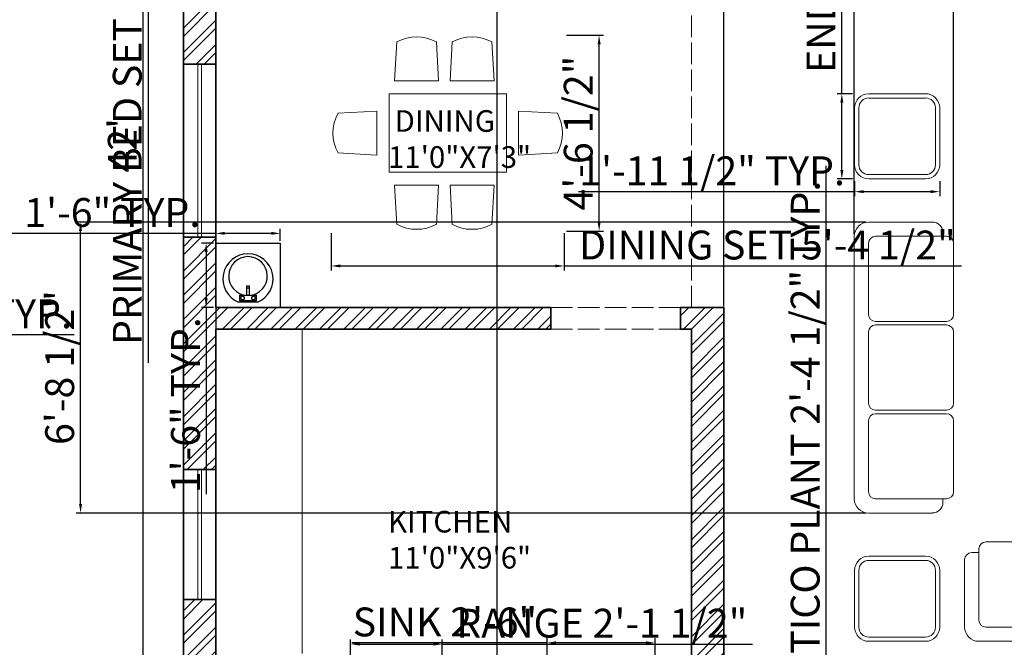
# Model space of a CAD drawing. Units: inches. Extents: x 3595 to 4516, y 2363 to 2965.
# Tile 7 of 12: x 4036 to 4309, y 2512 to 2686. Entities that reach past the tile are written whole.
import ezdxf

# ---------------------------------------------------------------- set-up
doc = ezdxf.new("R2010")
doc.units = ezdxf.units.IN
doc.linetypes.add('ACAD_ISO02W100', pattern=[15, 12, -3])
for name, color, linetype, lineweight in [('A-ANNO-DIMS', 2, 'Continuous', 18), ('A-AREA-IDEN', 7, 'Continuous', 18), ('A-FLOR-CASE', 9, 'Continuous', 18), ('A-FLOR-FIXT', 8, 'Continuous', 18), ('A-FURN', 43, 'Continuous', 18), ('A-GLAZ', 4, 'Continuous', 18), ('A-WALL', 7, 'Continuous', 35), ('A-WALL-OVHD', 7, 'ACAD_ISO02W100', 18)]:
    doc.layers.add(name, color=color, linetype=linetype, lineweight=lineweight)
doc.layers.add('A-WALL-PATT', color=251, linetype='Continuous', lineweight=13, true_color=0x636466)
doc.layers.add('SANTEH', color=7, linetype='Continuous')
doc.styles.get("Standard").update_dxf_attribs({"font": 'arial.ttf'})
doc.dimstyles.new('ISO-25', dxfattribs={"dimtxt": 8, "dimasz": 2.5, "dimexe": 1.25, "dimexo": 0.625, "dimtad": 1, "dimdec": 1, "dimlunit": 3, "dimtxsty": 'Standard', "dimcen": 2.5, "dimadec": 0, "dimazin": 0, "dimtfac": 1, "dimtdec": 1, "dimtmove": 0, "dimatfit": 3, "dimfxl": 1, "dimarcsym": 0})

# ---------------------------------------------------------------- blocks, each defined once
blk = doc.blocks.new('*D6')
at = {"layer": 'A-ANNO-DIMS', "color": 0, "lineweight": -2, "transparency": 16777216}
for p, q in [((4080.62, 2903.04), (4068.71, 2903.04)), ((4069.96, 2900.54), (4069.96, 2401.54)), ((4080.62, 2399.04), (4068.71, 2399.04))]:
    blk.add_line(p, q, dxfattribs=at)
at = {"layer": 'A-ANNO-DIMS', "color": 0, "transparency": 16777216}
for points in [[(4069.55, 2900.54), (4070.38, 2900.54), (4069.96, 2903.04)], [(4069.55, 2401.54), (4070.38, 2401.54), (4069.96, 2399.04)]]:
    blk.add_solid(points, dxfattribs=at)
at = {"layer": 'Defpoints', "color": 0, "transparency": 16777216}
for p in [(4081.24, 2903.04), (4069.96, 2399.04), (4081.24, 2399.04)]:
    blk.add_point(p, dxfattribs=at)
at = {"layer": 'A-ANNO-DIMS', "color": 0, "transparency": 16777216, "insert": (4065.32, 2651.04), "char_height": 8, "attachment_point": 5, "rotation": 90}
blk.add_mtext("42'", dxfattribs=at)
blk = doc.blocks.new('table-11')
at = {"color": 0, "linetype": 'ByBlock'}
for p, q in [((-1.122, 0.533), (-1.144, 0.134)), ((-0.716, 0.533), (-0.694, 0.134)), ((-0.554, 0.533), (-0.576, 0.134)), ((-0.148, 0.533), (-0.126, 0.134)), ((-1.144, 0.134), (-0.694, 0.134)), ((-0.576, 0.134), (-0.126, 0.134)), ((0, 0), (-1.2, 0)), ((-1.2, -0.8), (-1.2, 0)), ((0, -0.8), (0, 0)), ((-1.723, -0.197), (-1.324, -0.175)), ((-1.324, -0.625), (-1.324, -0.175)), ((0.523, -0.197), (0.124, -0.175)), ((0.124, -0.625), (0.124, -0.175)), ((-1.723, -0.603), (-1.324, -0.625)), ((0.523, -0.603), (0.124, -0.625)), ((0, -0.8), (-1.2, -0.8)), ((-1.144, -0.934), (-0.694, -0.934)), ((-1.122, -1.333), (-1.144, -0.934)), ((-0.716, -1.333), (-0.694, -0.934)), ((-0.576, -0.934), (-0.126, -0.934)), ((-0.554, -1.333), (-0.576, -0.934)), ((-0.148, -1.333), (-0.126, -0.934))]:
    blk.add_line(p, q, dxfattribs=at)
for centre, start, end in [((-0.919, 0.159), 61.4891, 118.5109), ((-0.351, 0.159), 61.4891, 118.5109), ((-1.349, -0.4), 151.4891, 208.5109), ((0.149, -0.4), 331.4891, 28.5109), ((-0.919, -0.959), 241.4891, 298.5109), ((-0.351, -0.959), 241.4891, 298.5109)]:
    blk.add_arc(centre, 0.425, start, end, dxfattribs=at)
blk = doc.blocks.new('r11')
at = {"layer": 'SANTEH', "ltscale": 5}
for p, q in [((0, 0), (600, 0)), ((0, -600), (0, 0)), ((600, 0), (600, -600)), ((210.5, -50), (389.5, -50)), ((210.5, -50), (210.5, -50)), ((223.8, -63.2), (376.2, -63.2)), ((223.8, -113.2), (223.8, -63.2)), ((232.7, -78.7), (249.2, -69.1)), ((232.7, -97.7), (232.7, -78.7)), ((249.2, -69.1), (265.7, -78.7)), ((265.7, -78.7), (265.7, -97.7)), ((334.3, -78.7), (350.8, -69.1)), ((334.3, -97.7), (334.3, -78.7)), ((350.8, -69.1), (367.3, -78.7)), ((367.3, -78.7), (367.3, -97.7)), ((376.2, -63.2), (376.2, -113.2)), ((376.2, -113.2), (223.8, -113.2)), ((249.2, -107.2), (232.7, -97.7)), ((265.7, -97.7), (249.2, -107.2)), ((288, -201.6), (288, -113.2)), ((312, -113.2), (312, -201.6)), ((350.8, -107.2), (334.3, -97.7)), ((367.3, -97.7), (350.8, -107.2)), ((312, -184.3), (288, -184.3)), ((312, -201.6), (288, -201.6)), ((600, -600), (0, -600))]:
    blk.add_line(p, q, dxfattribs=at)
for centre, radius, start, end in [((300, -266.2), 234, 112.50001, 67.49999), ((300, -293), 180.2, 93.8183, 86.1817)]:
    blk.add_arc(centre, radius, start, end, dxfattribs=at)
blk = doc.blocks.new('WIN-GLAZING-36IN')
for p, q in [((0, 1), (36, 1)), ((0, 0), (36, 0))]:
    blk.add_line(p, q)
blk = doc.blocks.new('WIN-GLAZING-48IN')
for p, q in [((0, 1), (48, 1)), ((0, 0), (48, 0))]:
    blk.add_line(p, q)
blk = doc.blocks.new('LOUNGE-ARMCHAIR')
for p, q in [((5.91, 27.56), (25.59, 27.56)), ((1.97, 24.61), (3.94, 24.61)), ((3.94, 5.91), (3.94, 25.59)), ((27.56, 25.59), (27.56, 5.91)), ((27.56, 24.61), (29.53, 24.61)), ((0, 3.94), (0, 22.64)), ((31.5, 22.64), (31.5, 3.94)), ((25.59, 3.94), (5.91, 3.94)), ((27.56, 0), (3.94, 0))]:
    blk.add_line(p, q)
for centre, radius, start, end in [((5.91, 25.59), 1.97, 90, 180), ((25.59, 25.59), 1.97, 360, 90), ((1.97, 22.64), 1.97, 90, 180), ((29.53, 22.64), 1.97, 360, 90), ((5.91, 5.91), 1.97, 180, 270), ((25.59, 5.91), 1.97, 270, 0), ((3.94, 3.94), 3.94, 180, 270), ((27.56, 3.94), 3.94, 270, 0)]:
    blk.add_arc(centre, radius, start, end)
blk = doc.blocks.new('LOUNGE-SIDE-TABLE')
for p, q in [((3.94, 23.62), (19.69, 23.62)), ((3.94, 22.44), (19.69, 22.44)), ((0, 3.94), (0, 19.69)), ((1.18, 3.94), (1.18, 19.69)), ((22.44, 19.69), (22.44, 3.94)), ((23.62, 19.69), (23.62, 3.94)), ((19.69, 1.18), (3.94, 1.18)), ((19.69, 0), (3.94, 0))]:
    blk.add_line(p, q)
for centre, radius, start, end in [((3.94, 19.69), 3.94, 90, 180), ((3.94, 19.69), 2.76, 90, 180), ((19.69, 19.69), 3.94, 360, 90), ((19.69, 19.69), 2.76, 360, 90), ((3.94, 3.94), 3.94, 180, 270), ((3.94, 3.94), 2.76, 180, 270), ((19.69, 3.94), 3.94, 270, 0), ((19.69, 3.94), 2.76, 270, 0)]:
    blk.add_arc(centre, radius, start, end)
blk = doc.blocks.new('*D104')
at = {"layer": 'A-ANNO-DIMS', "color": 0, "lineweight": -2, "transparency": 16777216}
for p, q in [((3994.89, 2606.92), (3994.89, 2597.29)), ((3995.89, 2606.92), (3995.89, 2597.29)), ((3992.39, 2598.54), (3989.89, 2598.54)), ((3994.89, 2598.54), (3995.89, 2598.54)), ((3998.39, 2598.54), (4050.91, 2598.54))]:
    blk.add_line(p, q, dxfattribs=at)
at = {"layer": 'A-ANNO-DIMS', "color": 0, "transparency": 16777216}
for points in [[(3992.39, 2598.96), (3992.39, 2598.13), (3994.89, 2598.54)], [(3998.39, 2598.96), (3998.39, 2598.13), (3995.89, 2598.54)]]:
    blk.add_solid(points, dxfattribs=at)
at = {"layer": 'Defpoints', "color": 0, "transparency": 16777216}
for p in [(3994.89, 2607.54), (3995.89, 2607.54), (3995.89, 2598.54)]:
    blk.add_point(p, dxfattribs=at)
at = {"layer": 'A-ANNO-DIMS', "color": 0, "transparency": 16777216, "insert": (4025.9, 2603.25), "char_height": 8, "attachment_point": 5}
blk.add_mtext('0\'-1" TYP.', dxfattribs=at)
blk = doc.blocks.new('*D115')
at = {"layer": 'A-ANNO-DIMS', "color": 0, "lineweight": -2, "transparency": 16777216}
for p, q in [((4183.24, 2696.92), (4183.24, 2690.89)), ((4219.24, 2696.92), (4219.24, 2690.89)), ((4183.24, 2692.14), (4033.6, 2692.14)), ((4216.74, 2692.14), (4185.74, 2692.14))]:
    blk.add_line(p, q, dxfattribs=at)
at = {"layer": 'A-ANNO-DIMS', "color": 0, "transparency": 16777216}
for points in [[(4185.74, 2692.56), (4185.74, 2691.73), (4183.24, 2692.14)], [(4216.74, 2692.56), (4216.74, 2691.73), (4219.24, 2692.14)]]:
    blk.add_solid(points, dxfattribs=at)
at = {"layer": 'Defpoints', "color": 0, "transparency": 16777216}
for p in [(4183.24, 2697.54), (4219.24, 2697.54), (4183.24, 2692.14)]:
    blk.add_point(p, dxfattribs=at)
at = {"layer": 'A-ANNO-DIMS', "color": 0, "transparency": 16777216, "insert": (4107.17, 2696.91), "char_height": 8, "attachment_point": 5}
blk.add_mtext('BEDROOM DOOR 3\'-0" TYP.', dxfattribs=at)
blk = doc.blocks.new('*D119')
at = {"layer": 'A-ANNO-DIMS', "color": 0, "lineweight": -2, "transparency": 16777216}
for p, q in [((4089.62, 2851.64), (4070.21, 2851.64)), ((4071.46, 2849.14), (4071.46, 2728.95)), ((4089.62, 2726.45), (4070.21, 2726.45)), ((4071.46, 2726.45), (4071.46, 2590.66))]:
    blk.add_line(p, q, dxfattribs=at)
at = {"layer": 'A-ANNO-DIMS', "color": 0, "transparency": 16777216}
for points in [[(4071.05, 2849.14), (4071.88, 2849.14), (4071.46, 2851.64)], [(4071.05, 2728.95), (4071.88, 2728.95), (4071.46, 2726.45)]]:
    blk.add_solid(points, dxfattribs=at)
at = {"layer": 'Defpoints', "color": 0, "transparency": 16777216}
for p in [(4090.24, 2851.64), (4071.46, 2726.45), (4090.24, 2726.45)]:
    blk.add_point(p, dxfattribs=at)
at = {"layer": 'A-ANNO-DIMS', "color": 0, "transparency": 16777216, "insert": (4066.7, 2657.3), "char_height": 8, "attachment_point": 5, "rotation": 90}
blk.add_mtext('PRIMARY BED SET 10\'-5"', dxfattribs=at)
blk = doc.blocks.new('*D121')
at = {"layer": 'A-ANNO-DIMS', "color": 0, "lineweight": -2, "transparency": 16777216}
for p, q in [((4122.3, 2626.62), (4122.3, 2616.3)), ((4186.94, 2626.62), (4186.94, 2616.3)), ((4124.8, 2617.55), (4184.44, 2617.55)), ((4186.94, 2617.55), (4297.26, 2617.55))]:
    blk.add_line(p, q, dxfattribs=at)
at = {"layer": 'A-ANNO-DIMS', "color": 0, "transparency": 16777216}
for points in [[(4124.8, 2617.97), (4124.8, 2617.14), (4122.3, 2617.55)], [(4184.44, 2617.97), (4184.44, 2617.14), (4186.94, 2617.55)]]:
    blk.add_solid(points, dxfattribs=at)
at = {"layer": 'Defpoints', "color": 0, "transparency": 16777216}
for p in [(4122.3, 2627.25), (4186.94, 2627.25), (4186.94, 2617.55)]:
    blk.add_point(p, dxfattribs=at)
at = {"layer": 'A-ANNO-DIMS', "color": 0, "transparency": 16777216, "insert": (4243.35, 2622.32), "char_height": 8, "attachment_point": 5}
blk.add_mtext('DINING SET 5\'-4 1/2"', dxfattribs=at)
blk = doc.blocks.new('*D122')
at = {"layer": 'A-ANNO-DIMS', "color": 0, "lineweight": -2, "transparency": 16777216}
for p, q in [((4187.56, 2681.58), (4197.88, 2681.58)), ((4196.63, 2629.75), (4196.63, 2679.08)), ((4187.56, 2627.25), (4197.88, 2627.25))]:
    blk.add_line(p, q, dxfattribs=at)
at = {"layer": 'A-ANNO-DIMS', "color": 0, "transparency": 16777216}
for points in [[(4196.22, 2679.08), (4197.05, 2679.08), (4196.63, 2681.58)], [(4196.22, 2629.75), (4197.05, 2629.75), (4196.63, 2627.25)]]:
    blk.add_solid(points, dxfattribs=at)
at = {"layer": 'Defpoints', "color": 0, "transparency": 16777216}
for p in [(4186.94, 2681.58), (4196.63, 2681.58), (4186.94, 2627.25)]:
    blk.add_point(p, dxfattribs=at)
at = {"layer": 'A-ANNO-DIMS', "color": 0, "transparency": 16777216, "insert": (4191.87, 2654.41), "char_height": 8, "attachment_point": 5, "rotation": 90}
blk.add_mtext('4\'-6 1/2"', dxfattribs=at)
blk = doc.blocks.new('*D129')
at = {"layer": 'A-ANNO-DIMS', "color": 0, "lineweight": -2, "transparency": 16777216}
for p, q in [((4090.24, 2626.59), (4001.44, 2626.59)), ((4090.24, 2624.54), (4090.24, 2627.84)), ((4105.61, 2626.59), (4092.74, 2626.59)), ((4108.11, 2624.54), (4108.11, 2627.84))]:
    blk.add_line(p, q, dxfattribs=at)
at = {"layer": 'A-ANNO-DIMS', "color": 0, "transparency": 16777216}
for points in [[(4092.74, 2627.01), (4092.74, 2626.18), (4090.24, 2626.59)], [(4105.61, 2627.01), (4105.61, 2626.18), (4108.11, 2626.59)]]:
    blk.add_solid(points, dxfattribs=at)
at = {"layer": 'Defpoints', "color": 0, "transparency": 16777216}
for p in [(4090.24, 2626.59), (4090.24, 2623.91), (4108.11, 2623.91)]:
    blk.add_point(p, dxfattribs=at)
at = {"layer": 'A-ANNO-DIMS', "color": 0, "transparency": 16777216, "insert": (4044.59, 2631.35), "char_height": 8, "attachment_point": 5}
blk.add_mtext('BASIN 1\'-6" TYP.', dxfattribs=at)
blk = doc.blocks.new('*D130')
at = {"layer": 'A-ANNO-DIMS', "color": 0, "lineweight": -2, "transparency": 16777216}
for p, q in [((4089.62, 2623.91), (4086.31, 2623.91)), ((4087.56, 2621.41), (4087.56, 2608.54)), ((4089.62, 2606.04), (4086.31, 2606.04)), ((4087.56, 2606.04), (4087.56, 2554.28))]:
    blk.add_line(p, q, dxfattribs=at)
at = {"layer": 'A-ANNO-DIMS', "color": 0, "transparency": 16777216}
for points in [[(4087.15, 2621.41), (4087.98, 2621.41), (4087.56, 2623.91)], [(4087.15, 2608.54), (4087.98, 2608.54), (4087.56, 2606.04)]]:
    blk.add_solid(points, dxfattribs=at)
at = {"layer": 'Defpoints', "color": 0, "transparency": 16777216}
for p in [(4090.24, 2623.91), (4087.56, 2606.04), (4090.24, 2606.04)]:
    blk.add_point(p, dxfattribs=at)
at = {"layer": 'A-ANNO-DIMS', "color": 0, "transparency": 16777216, "insert": (4082.85, 2578.91), "char_height": 8, "attachment_point": 5, "rotation": 90}
blk.add_mtext('1\'-6" TYP.', dxfattribs=at)
blk = doc.blocks.new('*D135')
at = {"layer": 'A-ANNO-DIMS', "color": 0, "lineweight": -2, "transparency": 16777216}
for p, q in [((4127.63, 2509.45), (4127.63, 2513.89)), ((4130.13, 2512.64), (4150.59, 2512.64)), ((4153.09, 2509.45), (4153.09, 2513.89)), ((4153.09, 2512.64), (4239.18, 2512.64))]:
    blk.add_line(p, q, dxfattribs=at)
at = {"layer": 'A-ANNO-DIMS', "color": 0, "transparency": 16777216}
for points in [[(4130.13, 2513.06), (4130.13, 2512.22), (4127.63, 2512.64)], [(4150.59, 2513.06), (4150.59, 2512.22), (4153.09, 2512.64)]]:
    blk.add_solid(points, dxfattribs=at)
at = {"layer": 'Defpoints', "color": 0, "transparency": 16777216}
for p in [(4153.09, 2512.64), (4127.63, 2508.82), (4153.09, 2508.82)]:
    blk.add_point(p, dxfattribs=at)
at = {"layer": 'A-ANNO-DIMS', "color": 0, "transparency": 16777216, "insert": (4197.38, 2517.4), "char_height": 8, "attachment_point": 5}
blk.add_mtext('RANGE 2\'-1 1/2"', dxfattribs=at)
blk = doc.blocks.new('*D137')
at = {"layer": 'A-ANNO-DIMS', "color": 0, "lineweight": -2, "transparency": 16777216}
for p, q in [((4182.18, 2512.99), (4128.01, 2512.99)), ((4182.18, 2509.12), (4182.18, 2514.24)), ((4209.68, 2512.99), (4184.68, 2512.99)), ((4212.18, 2509.12), (4212.18, 2514.24))]:
    blk.add_line(p, q, dxfattribs=at)
at = {"layer": 'A-ANNO-DIMS', "color": 0, "transparency": 16777216}
for points in [[(4184.68, 2513.41), (4184.68, 2512.58), (4182.18, 2512.99)], [(4209.68, 2513.41), (4209.68, 2512.58), (4212.18, 2512.99)]]:
    blk.add_solid(points, dxfattribs=at)
at = {"layer": 'Defpoints', "color": 0, "transparency": 16777216}
for p in [(4182.18, 2512.99), (4182.18, 2508.49), (4212.18, 2508.49)]:
    blk.add_point(p, dxfattribs=at)
at = {"layer": 'A-ANNO-DIMS', "color": 0, "transparency": 16777216, "insert": (4153.84, 2517.75), "char_height": 8, "attachment_point": 5}
blk.add_mtext('SINK 2\'-6"', dxfattribs=at)
blk = doc.blocks.new('*D141')
at = {"layer": 'A-ANNO-DIMS', "color": 0, "lineweight": -2, "transparency": 16777216}
for p, q in [((4264, 2665.33), (4264, 2807.49)), ((4266.92, 2665.33), (4262.75, 2665.33)), ((4264, 2644.21), (4264, 2662.83)), ((4266.92, 2641.71), (4262.75, 2641.71))]:
    blk.add_line(p, q, dxfattribs=at)
at = {"layer": 'A-ANNO-DIMS', "color": 0, "transparency": 16777216}
for points in [[(4263.59, 2662.83), (4264.42, 2662.83), (4264, 2665.33)], [(4263.59, 2644.21), (4264.42, 2644.21), (4264, 2641.71)]]:
    blk.add_solid(points, dxfattribs=at)
at = {"layer": 'Defpoints', "color": 0, "transparency": 16777216}
for p in [(4264, 2665.33), (4267.55, 2665.33), (4267.55, 2641.71)]:
    blk.add_point(p, dxfattribs=at)
at = {"layer": 'A-ANNO-DIMS', "color": 0, "transparency": 16777216, "insert": (4259.24, 2737.66), "char_height": 8, "attachment_point": 5, "rotation": 90}
blk.add_mtext('END TABLE 1\'-11 1/2" TYP.', dxfattribs=at)
blk = doc.blocks.new('*D142')
at = {"layer": 'A-ANNO-DIMS', "color": 0, "lineweight": -2, "transparency": 16777216}
for p, q in [((4267.55, 2641.08), (4267.55, 2636.91)), ((4291.17, 2641.08), (4291.17, 2636.91)), ((4267.55, 2638.16), (4190.93, 2638.16)), ((4288.67, 2638.16), (4270.05, 2638.16))]:
    blk.add_line(p, q, dxfattribs=at)
at = {"layer": 'A-ANNO-DIMS', "color": 0, "transparency": 16777216}
for points in [[(4270.05, 2638.58), (4270.05, 2637.75), (4267.55, 2638.16)], [(4288.67, 2638.58), (4288.67, 2637.75), (4291.17, 2638.16)]]:
    blk.add_solid(points, dxfattribs=at)
at = {"layer": 'Defpoints', "color": 0, "transparency": 16777216}
for p in [(4267.55, 2641.71), (4291.17, 2641.71), (4267.55, 2638.16)]:
    blk.add_point(p, dxfattribs=at)
at = {"layer": 'A-ANNO-DIMS', "color": 0, "transparency": 16777216, "insert": (4227.99, 2642.92), "char_height": 8, "attachment_point": 5}
blk.add_mtext('1\'-11 1/2" TYP.', dxfattribs=at)
blk = doc.blocks.new('*D145')
at = {"layer": 'A-ANNO-DIMS', "color": 0, "lineweight": -2, "transparency": 16777216}
for p, q in [((4259.64, 2481.4), (4259.64, 2645.3)), ((4255.95, 2481.4), (4260.89, 2481.4)), ((4259.64, 2455.16), (4259.64, 2478.9)), ((4255.95, 2452.66), (4260.89, 2452.66))]:
    blk.add_line(p, q, dxfattribs=at)
at = {"layer": 'A-ANNO-DIMS', "color": 0, "transparency": 16777216}
for points in [[(4259.22, 2478.9), (4260.06, 2478.9), (4259.64, 2481.4)], [(4259.22, 2455.16), (4260.06, 2455.16), (4259.64, 2452.66)]]:
    blk.add_solid(points, dxfattribs=at)
at = {"layer": 'Defpoints', "color": 0, "transparency": 16777216}
for p in [(4255.33, 2481.4), (4259.64, 2481.4), (4255.33, 2452.66)]:
    blk.add_point(p, dxfattribs=at)
at = {"layer": 'A-ANNO-DIMS', "color": 0, "transparency": 16777216, "insert": (4254.87, 2564.6), "char_height": 8, "attachment_point": 5, "rotation": 90}
blk.add_mtext('PORTICO PLANT 2\'-4 1/2" TYP.', dxfattribs=at)
blk = doc.blocks.new('*D163')
at = {"layer": 'A-ANNO-DIMS', "color": 0, "lineweight": -2, "transparency": 16777216}
for p, q in [((4267.47, 2626.41), (4267.47, 2932.84)), ((4295.03, 2624.44), (4295.03, 2932.84)), ((4269.97, 2931.59), (4292.53, 2931.59)), ((4295.03, 2931.59), (4338.82, 2931.59))]:
    blk.add_line(p, q, dxfattribs=at)
at = {"layer": 'A-ANNO-DIMS', "color": 0, "transparency": 16777216}
for points in [[(4269.97, 2932.01), (4269.97, 2931.18), (4267.47, 2931.59)], [(4292.53, 2932.01), (4292.53, 2931.18), (4295.03, 2931.59)]]:
    blk.add_solid(points, dxfattribs=at)
at = {"layer": 'Defpoints', "color": 0, "transparency": 16777216}
for p in [(4295.03, 2931.59), (4267.47, 2625.78), (4295.03, 2623.82)]:
    blk.add_point(p, dxfattribs=at)
at = {"layer": 'A-ANNO-DIMS', "color": 0, "transparency": 16777216, "insert": (4318.18, 2936.36), "char_height": 8, "attachment_point": 5}
blk.add_mtext('2\'-3 1/2"', dxfattribs=at)
blk = doc.blocks.new('*D164')
at = {"layer": 'A-ANNO-DIMS', "color": 0, "lineweight": -2, "transparency": 16777216}
for p, q in [((4270.78, 2629.72), (4051.44, 2629.72)), ((4052.69, 2551.51), (4052.69, 2627.22)), ((4270.78, 2549.01), (4051.44, 2549.01))]:
    blk.add_line(p, q, dxfattribs=at)
at = {"layer": 'A-ANNO-DIMS', "color": 0, "transparency": 16777216}
for points in [[(4052.28, 2627.22), (4053.11, 2627.22), (4052.69, 2629.72)], [(4052.28, 2551.51), (4053.11, 2551.51), (4052.69, 2549.01)]]:
    blk.add_solid(points, dxfattribs=at)
at = {"layer": 'Defpoints', "color": 0, "transparency": 16777216}
for p in [(4052.69, 2629.72), (4271.41, 2629.72), (4271.41, 2549.01)]:
    blk.add_point(p, dxfattribs=at)
at = {"layer": 'A-ANNO-DIMS', "color": 0, "transparency": 16777216, "insert": (4047.93, 2589.37), "char_height": 8, "attachment_point": 5, "rotation": 90}
blk.add_mtext('6\'-8 1/2"', dxfattribs=at)
blk = doc.blocks.new('*D167')
at = {"layer": 'A-ANNO-DIMS', "color": 0, "lineweight": -2, "transparency": 16777216}
for p, q in [((4231.24, 2606.67), (4231.24, 2932.84)), ((4267.47, 2626.41), (4267.47, 2932.84)), ((4233.74, 2931.59), (4264.97, 2931.59))]:
    blk.add_line(p, q, dxfattribs=at)
at = {"layer": 'A-ANNO-DIMS', "color": 0, "transparency": 16777216}
for points in [[(4233.74, 2932.01), (4233.74, 2931.18), (4231.24, 2931.59)], [(4264.97, 2932.01), (4264.97, 2931.18), (4267.47, 2931.59)]]:
    blk.add_solid(points, dxfattribs=at)
at = {"layer": 'Defpoints', "color": 0, "transparency": 16777216}
for p in [(4267.47, 2931.59), (4267.47, 2625.78), (4231.24, 2606.04)]:
    blk.add_point(p, dxfattribs=at)
at = {"layer": 'A-ANNO-DIMS', "color": 0, "transparency": 16777216, "insert": (4249.36, 2936.31), "char_height": 8, "attachment_point": 5}
blk.add_mtext('3\'-0"', dxfattribs=at)
blk = doc.blocks.new('*D170')
at = {"layer": 'A-ANNO-DIMS', "color": 0, "lineweight": -2, "transparency": 16777216}
for p, q in [((4090.24, 2875.42), (4090.24, 2369.24)), ((4168.24, 2875.42), (4168.24, 2369.24)), ((4092.74, 2370.49), (4165.74, 2370.49))]:
    blk.add_line(p, q, dxfattribs=at)
at = {"layer": 'A-ANNO-DIMS', "color": 0, "transparency": 16777216}
for points in [[(4092.74, 2370.91), (4092.74, 2370.08), (4090.24, 2370.49)], [(4165.74, 2370.91), (4165.74, 2370.08), (4168.24, 2370.49)]]:
    blk.add_solid(points, dxfattribs=at)
at = {"layer": 'Defpoints', "color": 0, "transparency": 16777216}
for p in [(4090.24, 2876.04), (4168.24, 2876.04), (4168.24, 2370.49)]:
    blk.add_point(p, dxfattribs=at)
at = {"layer": 'A-ANNO-DIMS', "color": 0, "transparency": 16777216, "insert": (4129.24, 2375.2), "char_height": 8, "attachment_point": 5}
blk.add_mtext('6\'-6"', dxfattribs=at)

msp = doc.modelspace()

# ---------------------------------------------------------------- hatches: boundary and pattern name
at = {"layer": 'A-WALL-PATT'}
h = msp.add_hatch(dxfattribs=at)
h.set_pattern_fill('ANSI32', color=256, scale=0.5)
h.set_pattern_definition([(45, (441.351, 0), (-3.367596, 3.367596), []), (45, (443.596, 0), (-3.367596, 3.367596), [])])
h.paths.add_polyline_path([(4081.24, 2756.04), (4090.24, 2756.04), (4090.24, 2894.04), (4168.24, 2894.04), (4168.24, 2903.04), (4081.24, 2903.04)])
h.paths.add_polyline_path([(4216.24, 2903.04), (4216.24, 2894.04), (4222.24, 2894.04), (4222.24, 2792.04), (4231.24, 2792.04), (4231.24, 2894.04), (4241.74, 2894.04), (4241.74, 2903.04)])
h.paths.add_polyline_path([(4324.24, 2894.04), (4324.24, 2903.04), (4277.74, 2903.04), (4277.74, 2894.04), (4288.24, 2894.04), (4288.24, 2798.04), (4261.24, 2798.04), (4261.24, 2792.04), (4288.24, 2792.04), (4288.24, 2756.04), (4222.24, 2756.04), (4222.24, 2702.04), (4219.24, 2702.04), (4219.24, 2693.04), (4241.74, 2693.04), (4241.74, 2702.04), (4231.24, 2702.04), (4231.24, 2750.04), (4288.24, 2750.04), (4288.24, 2702.04), (4277.74, 2702.04), (4277.74, 2693.04), (4393.24, 2693.04), (4393.24, 2702.04), (4294.24, 2702.04), (4294.24, 2840.04), (4396.24, 2840.04), (4396.24, 2846.04), (4294.24, 2846.04), (4294.24, 2894.04)])
h.paths.add_polyline_path([(4390.24, 2894.04), (4390.24, 2876.04), (4396.24, 2876.04), (4396.24, 2894.04), (4432.24, 2894.04), (4432.24, 2795.04), (4441.24, 2795.04), (4441.24, 2903.04), (4360.24, 2903.04), (4360.24, 2894.04)])
h.paths.add_polyline_path([(4090.24, 2693.04), (4183.24, 2693.04), (4183.24, 2702.04), (4090.24, 2702.04), (4090.24, 2708.04), (4081.24, 2708.04), (4081.24, 2673.54), (4090.24, 2673.54)])
h.paths.add_polyline_path([(4090.24, 2600.04), (4183.24, 2600.04), (4183.24, 2606.04), (4090.24, 2606.04), (4090.24, 2625.54), (4081.24, 2625.54), (4081.24, 2561.04), (4090.24, 2561.04)])
h.paths.add_polyline_path([(4081.24, 2399.04), (4231.24, 2399.04), (4231.24, 2405.04), (4090.24, 2405.04), (4090.24, 2477.04), (4180.24, 2477.04), (4180.24, 2486.04), (4090.24, 2486.04), (4090.24, 2525.04), (4081.24, 2525.04)])
h.paths.add_polyline_path([(4231.24, 2486.04), (4231.24, 2606.04), (4219.24, 2606.04), (4219.24, 2600.04), (4222.24, 2600.04), (4222.24, 2486.04), (4216.24, 2486.04), (4216.24, 2477.04), (4273.24, 2477.04), (4273.24, 2486.04)])
h.paths.add_polyline_path([(4339.24, 2486.04), (4339.24, 2477.04), (4381.24, 2477.04), (4381.24, 2486.04)])
h.paths.add_polyline_path([(4432.24, 2486.04), (4429.24, 2486.04), (4429.24, 2477.04), (4441.24, 2477.04), (4441.24, 2511.54), (4432.24, 2511.54)])
h.paths.add_polyline_path([(4432.24, 2571.54), (4441.24, 2571.54), (4441.24, 2607.54), (4432.24, 2607.54)])
h.paths.add_polyline_path([(4441.24, 2747.04), (4432.24, 2747.04), (4432.24, 2702.04), (4429.24, 2702.04), (4429.24, 2693.04), (4432.24, 2693.04), (4432.24, 2667.54), (4441.24, 2667.54)])

# ---------------------------------------------------------------- linework, layer by layer
at = {"layer": 'A-FLOR-CASE'}
msp.add_line((4114.24, 2510.04), (4114.24, 2600.04), dxfattribs=at)
at = {"layer": 'A-FURN'}
for p, q in [((4271.41, 2629.72), (4289.12, 2629.72)), ((4292.08, 2626.77), (4292.08, 2625.78)), ((4267.47, 2552.95), (4267.47, 2625.78)), ((4271.41, 2604.13), (4271.41, 2623.82)), ((4273.38, 2625.78), (4293.06, 2625.78)), ((4295.03, 2623.82), (4295.03, 2604.13)), ((4293.06, 2602.16), (4273.38, 2602.16)), ((4271.41, 2579.52), (4271.41, 2599.21)), ((4273.38, 2601.18), (4293.06, 2601.18)), ((4295.03, 2599.21), (4295.03, 2579.52)), ((4293.06, 2577.56), (4273.38, 2577.56)), ((4271.41, 2554.92), (4271.41, 2574.6)), ((4273.38, 2576.57), (4293.06, 2576.57)), ((4295.03, 2574.6), (4295.03, 2554.92)), ((4293.06, 2552.95), (4273.38, 2552.95)), ((4292.08, 2552.95), (4292.08, 2551.97)), ((4289.12, 2549.01), (4271.41, 2549.01))]:
    msp.add_line(p, q, dxfattribs=at)
for centre, radius, start, end in [((4271.41, 2625.78), 3.94, 90, 180), ((4289.12, 2626.77), 2.95, 360, 90), ((4273.38, 2623.82), 1.97, 90, 180), ((4293.06, 2623.82), 1.97, 360, 90), ((4273.38, 2604.13), 1.97, 180, 270), ((4293.06, 2604.13), 1.97, 270, 0), ((4273.38, 2599.21), 1.97, 90, 180), ((4293.06, 2599.21), 1.97, 360, 90), ((4273.38, 2579.52), 1.97, 180, 270), ((4293.06, 2579.52), 1.97, 270, 0), ((4273.38, 2574.6), 1.97, 90, 180), ((4293.06, 2574.6), 1.97, 360, 90), ((4271.41, 2552.95), 3.94, 180, 270), ((4273.38, 2554.92), 1.97, 180, 270), ((4293.06, 2554.92), 1.97, 270, 0), ((4289.12, 2551.97), 2.95, 270, 0)]:
    msp.add_arc(centre, radius, start, end, dxfattribs=at)
at = {"layer": 'A-WALL'}
for p, q in [((4090.24, 2606.04), (4090.24, 2693.04)), ((4081.24, 2673.54), (4090.24, 2673.54)), ((4081.24, 2625.54), (4090.24, 2625.54)), ((4090.24, 2606.04), (4183.24, 2606.04)), ((4183.24, 2606.04), (4183.24, 2600.04)), ((4219.24, 2606.04), (4231.24, 2606.04)), ((4219.24, 2606.04), (4219.24, 2600.04)), ((4231.24, 2486.04), (4231.24, 2606.04)), ((4090.24, 2600.04), (4183.24, 2600.04)), ((4090.24, 2486.04), (4090.24, 2600.04)), ((4219.24, 2600.04), (4222.24, 2600.04)), ((4222.24, 2486.04), (4222.24, 2600.04)), ((4090.24, 2561.04), (4081.24, 2561.04)), ((4090.24, 2525.04), (4081.24, 2525.04))]:
    msp.add_line(p, q, dxfattribs=at)
msp.add_lwpolyline([(4231.24, 2399.04), (4081.24, 2399.04), (4081.24, 2903.04), (4441.24, 2903.04), (4441.24, 2477.04)], dxfattribs=at)
at = {"layer": 'A-WALL-OVHD', "ltscale": 0.5}
for p, q in [((4222.24, 2606.04), (4222.24, 2693.04)), ((4231.24, 2606.04), (4231.24, 2693.04)), ((4183.24, 2606.04), (4219.24, 2606.04)), ((4183.24, 2600.04), (4219.24, 2600.04))]:
    msp.add_line(p, q, dxfattribs=at)

# ---------------------------------------------------------------- block references
at = {"layer": 'A-FLOR-FIXT', "xscale": 0.0297800069284724, "yscale": 0.0297800069284724, "zscale": 0.0297800069284724, "rotation": 180}
msp.add_blockref('r11', (4108.11, 2606.04), dxfattribs=at)
at = {"layer": 'A-FURN', "xscale": 27.1273966238569, "yscale": 27.1273966238569, "zscale": 27.1273966238569}
msp.add_blockref('table-11', (4170.89, 2665.26), dxfattribs=at)
at = {"layer": 'A-FURN', "rotation": 90.00000000011806}
msp.add_blockref('LOUNGE-SIDE-TABLE', (4291.17, 2641.71), dxfattribs=at)
at = {"layer": 'A-FURN'}
for name, p in [('LOUNGE-ARMCHAIR', (4298.08, 2513.41)), ('LOUNGE-SIDE-TABLE', (4267.55, 2513.41))]:
    msp.add_blockref(name, p, dxfattribs=at)
at = {"layer": 'A-GLAZ'}
for name, p, rotation in [('WIN-GLAZING-48IN', (4085.24, 2673.54), 270), ('WIN-GLAZING-36IN', (4085.24, 2561.04), 270.0000000000014)]:
    msp.add_blockref(name, p, dxfattribs=dict(at, rotation=rotation))

# ---------------------------------------------------------------- texts
at = {"layer": 'A-AREA-IDEN', "char_height": 6, "attachment_point": 1}
for s, insert in [('{\\fTimes New Roman|b0|i0|c0|p18; DINING\\P11\'0"X7\'3"}', (4138.03, 2660.77)), ('{\\fTimes New Roman|b0|i0|c0|p18;KITCHEN\\P11\'0"X9\'6"}', (4138.03, 2549.6))]:
    msp.add_mtext_dynamic_manual_height_columns(s, width=67.3508, gutter_width=12.5, heights=[0], dxfattribs=dict(at, insert=insert))

# ---------------------------------------------------------------- dimensions: what is measured, and where the dimension line sits
at = {"layer": 'A-ANNO-DIMS'}
for base, p1, p2, picture, middle in [((4295.03, 2931.59), (4267.47, 2625.78), (4295.03, 2623.82), '*D163', (4318.18, 2936.36)), ((4267.47, 2931.59), (4231.24, 2606.04), (4267.47, 2625.78), '*D167', (4249.36, 2936.31)), ((4168.24, 2370.49), (4090.24, 2876.04), (4168.24, 2876.04), '*D170', (4129.24, 2375.2))]:
    dim = msp.add_linear_dim(base=base, p1=p1, p2=p2, dimstyle='ISO-25', override={"dimdec": 1, "dimlfac": 1, "dimrnd": 0, "dimzin": 1, "dimdsep": 46, "dimlunit": 4, "dimfrac": 2}, dxfattribs=at)
    dim.commit()
    dim.dimension.update_dxf_attribs({"geometry": picture, "text_midpoint": middle})
for base, p1, p2, override, picture, middle in [((4069.96, 2399.04), (4081.24, 2903.04), (4081.24, 2399.04), {"dimclrd": 0, "dimclre": 0, "dimclrt": 0}, '*D6', (4065.32, 2651.04)), ((4196.63, 2681.58), (4186.94, 2627.25), (4186.94, 2681.58), {"dimdec": 1, "dimlfac": 1, "dimrnd": 0, "dimzin": 1, "dimdsep": 46, "dimlunit": 4, "dimfrac": 2}, '*D122', (4191.87, 2654.41)), ((4052.69, 2629.72), (4271.41, 2549.01), (4271.41, 2629.72), {"dimdec": 1, "dimlfac": 1, "dimrnd": 0, "dimzin": 1, "dimdsep": 46, "dimlunit": 4, "dimfrac": 2}, '*D164', (4047.93, 2589.37))]:
    dim = msp.add_linear_dim(base=base, p1=p1, p2=p2, angle=90, dimstyle='ISO-25', override=override, dxfattribs=at)
    dim.commit()
    dim.dimension.update_dxf_attribs({"geometry": picture, "text_midpoint": middle})
for base, p1, p2, angle, text, picture, middle in [((4071.46, 2726.45), (4090.24, 2851.64), (4090.24, 2726.45), 270, 'PRIMARY BED SET <>', '*D119', (4066.7, 2657.3)), ((4264, 2665.33), (4267.55, 2641.71), (4267.55, 2665.33), 90, 'END TABLE <> TYP.', '*D141', (4259.24, 2737.66)), ((4183.24, 2692.14), (4219.24, 2697.54), (4183.24, 2697.54), 180, 'BEDROOM DOOR <> TYP.', '*D115', (4107.17, 2696.91)), ((4267.55, 2638.16), (4291.17, 2641.71), (4267.55, 2641.71), 180, '<> TYP.', '*D142', (4227.99, 2642.92)), ((4090.24, 2626.59), (4108.11, 2623.91), (4090.24, 2623.91), 180, 'BASIN <> TYP.', '*D129', (4044.59, 2631.35)), ((4259.64, 2481.4), (4255.33, 2452.66), (4255.33, 2481.4), 90, 'PORTICO PLANT <> TYP.', '*D145', (4254.87, 2564.6)), ((4087.56, 2606.04), (4090.24, 2623.91), (4090.24, 2606.04), 270, '<> TYP.', '*D130', (4082.85, 2578.91)), ((4182.18, 2512.99), (4212.18, 2508.49), (4182.18, 2508.49), 180, 'SINK <>', '*D137', (4153.84, 2517.75))]:
    dim = msp.add_linear_dim(base=base, p1=p1, p2=p2, angle=angle, text=text, dimstyle='ISO-25', override={"dimdec": 1, "dimlfac": 1, "dimrnd": 0, "dimzin": 1, "dimdsep": 46, "dimlunit": 4, "dimfrac": 2}, dxfattribs=at)
    dim.commit()
    dim.dimension.update_dxf_attribs({"geometry": picture, "text_midpoint": middle})
for base, p1, p2, text, picture, middle in [((4186.94, 2617.55), (4122.3, 2627.25), (4186.94, 2627.25), 'DINING SET <>', '*D121', (4243.35, 2622.32)), ((3995.89, 2598.54), (3994.89, 2607.54), (3995.89, 2607.54), '<> TYP.', '*D104', (4025.9, 2603.25)), ((4153.09, 2512.64), (4127.63, 2508.82), (4153.09, 2508.82), 'RANGE <>', '*D135', (4197.38, 2517.4))]:
    dim = msp.add_linear_dim(base=base, p1=p1, p2=p2, text=text, dimstyle='ISO-25', override={"dimdec": 1, "dimlfac": 1, "dimrnd": 0, "dimzin": 1, "dimdsep": 46, "dimlunit": 4, "dimfrac": 2}, dxfattribs=at)
    dim.commit()
    dim.dimension.update_dxf_attribs({"geometry": picture, "text_midpoint": middle})

doc.saveas('drawing.dxf')
